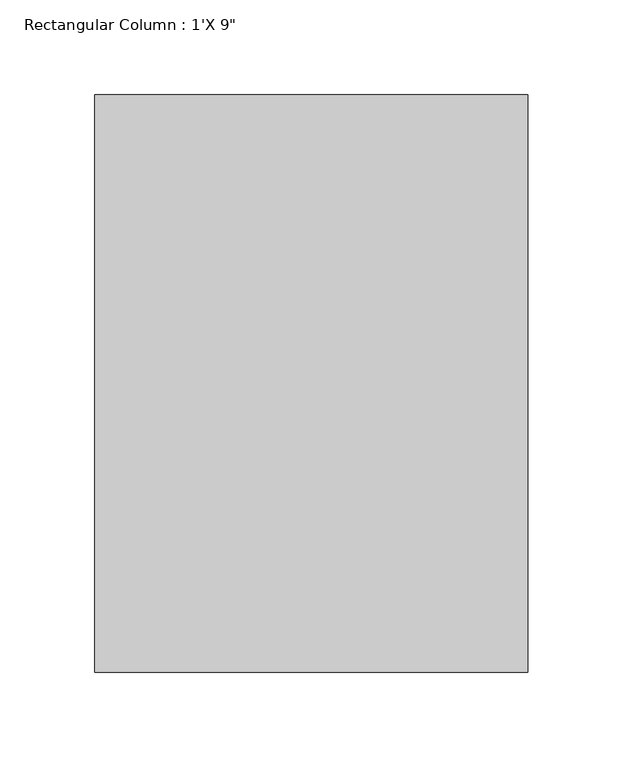
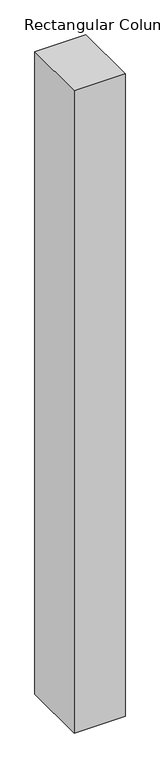
"""IFC4 building model written with IfcOpenShell, lengths in millimetres: column geometry."""

from ifc_helpers import new_model, si_unit, frame, origin, place, context, project, spatial, polyline, outline, extrude, source, transform, mapped, element, save


def column_68c8e778(model_context):
    return source(origin(), model_context, "Body", "SweptSolid", [
        extrude(outline(polyline([(114.3, 152.4), (114.3, -152.4), (-114.3, -152.4), (-114.3, 152.4), (114.3, 152.4)])), frame((0.0, 0.0, 28803.6), z_axis=(0.0, 0.0, 1.0), x_axis=(1.0, 0.0, 0.0)), (0.0, 0.0, 1.0), 3048.0),
    ])


if __name__ == "__main__":
    model = new_model("IFC4")
    model_context = context("Model", 3, world=origin())
    ifc_project = project(units=[si_unit("LENGTHUNIT", "METRE", prefix="MILLI")], contexts=[model_context])
    site = spatial("IfcSite", under=ifc_project)
    building = spatial("IfcBuilding", under=site)
    placement = place(None, origin())
    column_shape = column_68c8e778(model_context)
    element("IfcColumn", 1, ObjectType="Rectangular Column : 1'X 9\"", at=placement, inside=building, context=model_context, shape_type="MappedRepresentation", body=[
        mapped(column_shape, transform((0.0, 0.0, 0.0), x_axis=(1.0, 0.0, 0.0), y_axis=(0.0, 1.0, 0.0), z_axis=(0.0, 0.0, 1.0))),
    ])
    save(model, "model.ifc")

# Revit data of these elements
# Type "Rectangular Column : 1'X 9\""
#   Assembly Code = "B1010200"
#   Depth = 1' - 0"
#   Offset Base = 0' - 0"
#   Offset Top = 0' - 0"
#   Width = 0' - 9"
#   Material = none
